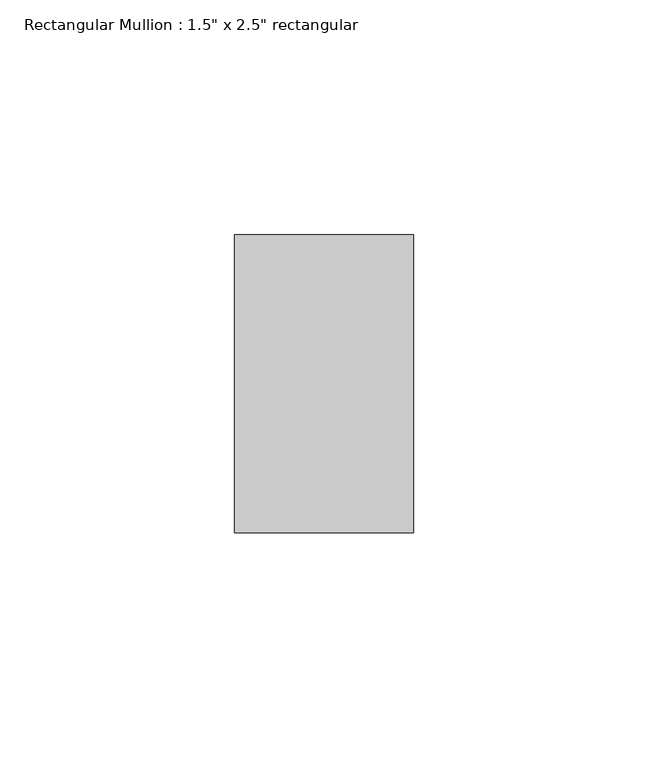
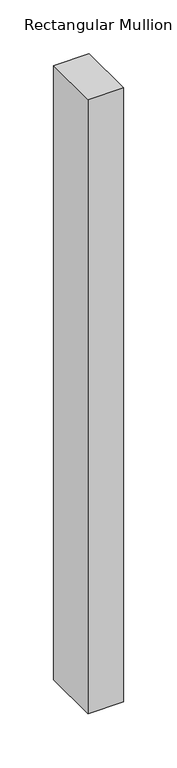
"""IFC4 building model written with IfcOpenShell, lengths in millimetres: member geometry."""

from ifc_helpers import new_model, si_unit, frame, origin, place, context, project, spatial, polyline, outline, extrude, source, transform, mapped, element, save


def member_57040902(model_context):
    return source(origin(), model_context, "Body", "SweptSolid", [
        extrude(outline(polyline([(0.0, 31.75), (0.0, -31.75), (-38.1, -31.75), (-38.1, 31.75), (0.0, 31.75)])), frame((0.0, 0.0, -696.6966705), z_axis=(0.0, 0.0, 1.0), x_axis=(1.0, 0.0, 0.0)), (0.0, 0.0, 1.0), 696.6966705),
    ])


if __name__ == "__main__":
    model = new_model("IFC4")
    model_context = context("Model", 3, world=origin())
    ifc_project = project(units=[si_unit("LENGTHUNIT", "METRE", prefix="MILLI")], contexts=[model_context])
    site = spatial("IfcSite", under=ifc_project)
    building = spatial("IfcBuilding", under=site)
    placement = place(None, origin())
    member_shape = member_57040902(model_context)
    element("IfcMember", 1, ObjectType="Rectangular Mullion : 1.5\" x 2.5\" rectangular", at=placement, inside=building, context=model_context, shape_type="MappedRepresentation", body=[
        mapped(member_shape, transform((0.0, 0.0, 0.0), x_axis=(1.0, 0.0, 0.0), y_axis=(0.0, 1.0, 0.0), z_axis=(0.0, 0.0, 1.0))),
    ])
    save(model, "model.ifc")

# Revit data of these elements
# Type "Rectangular Mullion : 1.5\" x 2.5\" rectangular"
#   built-in parameter 1007304 = 0.208333 (stored number, unit not read)
#   built-in parameter 1007301 = 0.0625 (stored number, unit not read)
#   built-in parameter 1007300 = 0.0625 (stored number, unit not read)
# Element 1 (IfcMember, "Rectangular Mullion : 1.5\" x 2.5\" rectangular")
#   Materials on its faces: "Damp-proofing"
# Materials
#   "Damp-proofing": class "Generic", colour RGB 127 127 127, transparency 0, Description = "Damp-proofing", Cost = 0
